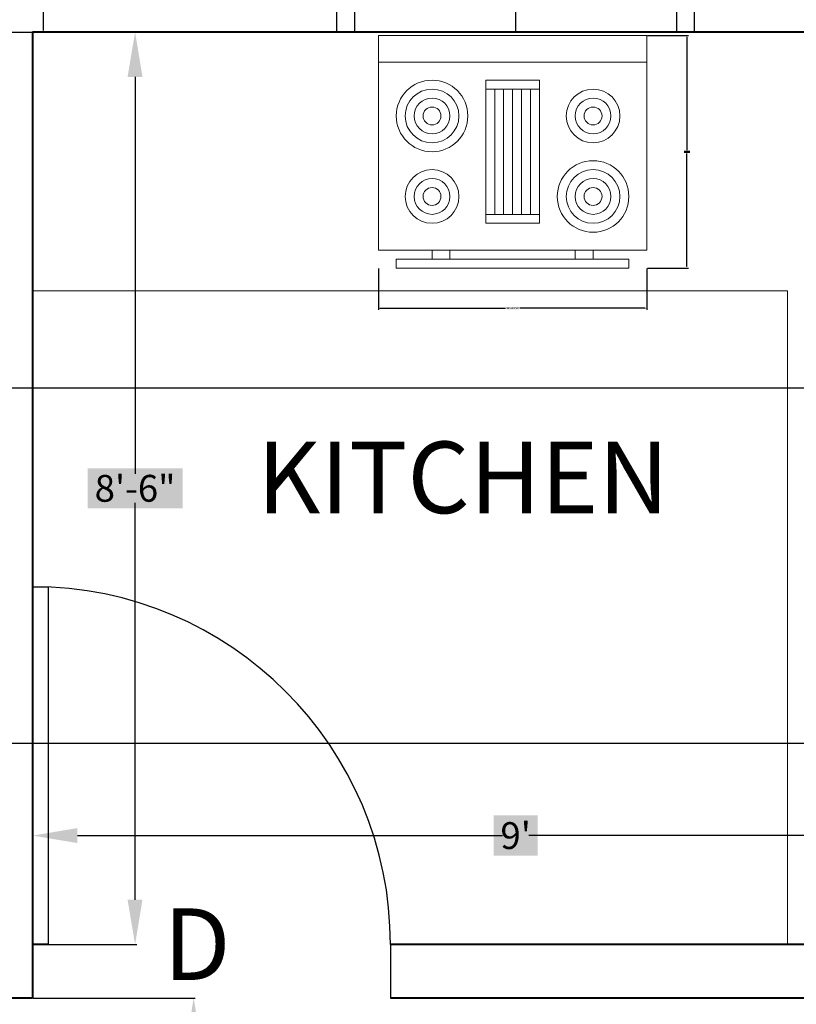
# Model space of a CAD drawing. Units: inches. Extents: x -301 to 715, y -607 to 364.
# Tile 118 of 141: x 14 to 101, y 192 to 303. Entities that reach past the tile are written whole.
import ezdxf

# ---------------------------------------------------------------- set-up
doc = ezdxf.new("R2010")
doc.units = ezdxf.units.IN
doc.header["$MEASUREMENT"] = 0
for name, color, linetype, lineweight in [('A-ANNO-DIMS', 2, 'Continuous', 18), ('A-ANNO-TEXT', 4, 'Continuous', 18), ('A-AREA-IDEN', 220, 'Continuous', 25), ('A-DOOR', 4, 'Continuous', 25), ('A-EQPM', 8, 'Continuous', 18), ('A-FLOR-CASE', 8, 'Continuous', 18), ('A-GLAZ', 2, 'Continuous', 25), ('A-WALL', 3, 'Continuous', 40)]:
    doc.layers.add(name, color=color, linetype=linetype, lineweight=lineweight)
doc.styles.get("Standard").update_dxf_attribs({"font": 'arial.ttf'})
doc.dimstyles.get("Standard").update_dxf_attribs({"dimtxt": 0.18, "dimasz": 0.18, "dimexe": 0.18, "dimexo": 0.0625, "dimgap": 0.09, "dimtad": 0, "dimtih": 1, "dimtoh": 1, "dimdec": 1, "dimzin": 0, "dimdsep": 46, "dimlunit": 4, "dimtxsty": 'Standard', "dimcen": 0.09, "dimclrd": 3, "dimclre": 4, "dimclrt": 6, "dimadec": 0, "dimazin": 0, "dimtfac": 1, "dimtdec": 1, "dimtofl": 0, "dimtmove": 0, "dimatfit": 3, "dimfxl": 1, "dimtfill": 2, "dimtfillclr": 51, "dimtolj": 1, "dimtzin": 0, "dimarcsym": 0})

# ---------------------------------------------------------------- blocks, each defined once
blk = doc.blocks.new('*U6')
for p, q in [((0, 0), (0, -6)), ((40, 0), (40, -6))]:
    blk.add_line(p, q)
blk.add_lwpolyline([(0, 0), (0, 40), (1.75, 40), (1.75, 0)], close=True)
blk.add_arc((0, 0), 40, 0, 90)
blk = doc.blocks.new('Range-Oven - 30 in top')
for p, q in [((0, -3), (30, -3)), ((12, -6), (18, -6)), ((13, -20), (13, -6)), ((14, -6), (14, -20)), ((15, -20), (15, -6)), ((16, -6), (16, -20)), ((17, -20), (17, -6)), ((18, -20), (12, -20)), ((6, -24), (6, -25)), ((8, -25), (8, -24)), ((22, -25), (22, -24)), ((24, -24), (24, -25))]:
    blk.add_line(p, q)
for points in [[(0, -24), (0, 0), (30, 0), (30, -24)], [(12, -21), (12, -5), (18, -5), (18, -21)], [(2, -26), (2, -25), (28, -25), (28, -26)]]:
    blk.add_lwpolyline(points, close=True)
for centre, radius in [((6, -9), 4), ((6, -9), 3), ((24, -9), 3), ((6, -9), 2), ((24, -9), 2), ((6, -9), 1), ((24, -9), 1), ((24, -18), 4), ((6, -18), 3), ((24, -18), 3), ((6, -18), 2), ((24, -18), 2), ((6, -18), 1), ((24, -18), 1)]:
    blk.add_circle(centre, radius)
blk = doc.blocks.new('*D49')
at = {"layer": 'A-ANNO-DIMS', "color": 0, "lineweight": -2, "transparency": 16777216}
for p, q in [((15.96, 193.18), (34.08, 193.18)), ((33.9, 188.18), (33.9, 93.3)), ((33.9, -4.82), (33.9, 90.06)), ((21.96, -9.82), (34.08, -9.82))]:
    blk.add_line(p, q, dxfattribs=at)
at = {"layer": 'A-ANNO-DIMS', "color": 0, "transparency": 16777216}
for points in [[(33.07, 188.18), (34.74, 188.18), (33.9, 193.18)], [(33.07, -4.82), (34.74, -4.82), (33.9, -9.82)]]:
    blk.add_solid(points, dxfattribs=at)
at = {"layer": 'Defpoints', "color": 0, "transparency": 16777216}
for p in [(15.9, 193.18), (33.9, 193.18), (21.9, -9.82)]:
    blk.add_point(p, dxfattribs=at)
at = {"layer": 'A-ANNO-DIMS', "color": 0, "transparency": 16777216, "insert": (33.9, 91.68), "char_height": 3, "attachment_point": 5, "bg_fill": 1, "box_fill_scale": 1.25, "bg_fill_color": 51, "bg_fill_transparency": 0}
blk.add_mtext('\\A1;16\'-11"', dxfattribs=at)
blk = doc.blocks.new('*D50')
at = {"layer": 'A-ANNO-DIMS', "color": 0, "lineweight": -2, "transparency": 16777216}
for p, q in [((15.9, 199.83), (15.9, 211.53)), ((123.9, 199.24), (123.9, 211.53)), ((20.9, 211.35), (68.43, 211.35)), ((118.9, 211.35), (71.37, 211.35))]:
    blk.add_line(p, q, dxfattribs=at)
at = {"layer": 'A-ANNO-DIMS', "color": 0, "transparency": 16777216}
for points in [[(20.9, 212.19), (20.9, 210.52), (15.9, 211.35)], [(118.9, 212.19), (118.9, 210.52), (123.9, 211.35)]]:
    blk.add_solid(points, dxfattribs=at)
at = {"layer": 'Defpoints', "color": 0, "transparency": 16777216}
for p in [(15.9, 211.35), (15.9, 199.77), (123.9, 199.18)]:
    blk.add_point(p, dxfattribs=at)
at = {"layer": 'A-ANNO-DIMS', "color": 0, "transparency": 16777216, "insert": (69.9, 211.35), "char_height": 3, "attachment_point": 5, "bg_fill": 1, "box_fill_scale": 1.25, "bg_fill_color": 51, "bg_fill_transparency": 0}
blk.add_mtext("\\A1;9'", dxfattribs=at)
blk = doc.blocks.new('*D51')
at = {"layer": 'A-ANNO-DIMS', "color": 0, "lineweight": -2, "transparency": 16777216}
for p, q in [((15.96, 301.18), (27.53, 301.18)), ((27.35, 296.18), (27.35, 251.8)), ((27.35, 204.18), (27.35, 248.56)), ((15.96, 199.18), (27.53, 199.18))]:
    blk.add_line(p, q, dxfattribs=at)
at = {"layer": 'A-ANNO-DIMS', "color": 0, "transparency": 16777216}
for points in [[(26.51, 296.18), (28.18, 296.18), (27.35, 301.18)], [(26.51, 204.18), (28.18, 204.18), (27.35, 199.18)]]:
    blk.add_solid(points, dxfattribs=at)
at = {"layer": 'Defpoints', "color": 0, "transparency": 16777216}
for p in [(15.9, 301.18), (15.9, 199.18), (27.35, 199.18)]:
    blk.add_point(p, dxfattribs=at)
at = {"layer": 'A-ANNO-DIMS', "color": 0, "transparency": 16777216, "insert": (27.35, 250.18), "char_height": 3, "attachment_point": 5, "bg_fill": 1, "box_fill_scale": 1.25, "bg_fill_color": 51, "bg_fill_transparency": 0}
blk.add_mtext('\\A1;8\'-6"', dxfattribs=at)
blk = doc.blocks.new('WIN-36-PLAN')
for p, q in [((0, 0), (0, 9)), ((2, 0), (2, 9)), ((20, 0), (20, 9)), ((38, 0), (38, 9)), ((40, 0), (40, 9)), ((2, 5.5), (38, 5.5)), ((2, 3.5), (38, 3.5))]:
    blk.add_line(p, q)
blk = doc.blocks.new('*D123')
at = {"layer": 'A-ANNO-DIMS', "color": 4, "lineweight": -2, "transparency": 16777216}
for p, q in [((9.96, 328.18), (17.28, 328.18)), ((9.96, 301.18), (17.28, 301.18))]:
    blk.add_line(p, q, dxfattribs=at)
at = {"layer": 'A-ANNO-DIMS', "color": 3, "lineweight": -2, "transparency": 16777216}
for p, q in [((17.1, 328), (17.1, 314.86)), ((17.1, 301.36), (17.1, 314.5))]:
    blk.add_line(p, q, dxfattribs=at)
at = {"layer": 'A-ANNO-DIMS', "color": 3, "transparency": 16777216}
for points in [[(17.07, 328), (17.13, 328), (17.1, 328.18)], [(17.07, 301.36), (17.13, 301.36), (17.1, 301.18)]]:
    blk.add_solid(points, dxfattribs=at)
at = {"layer": 'Defpoints', "color": 0, "transparency": 16777216}
for p in [(9.9, 328.18), (9.9, 301.18), (17.1, 301.18)]:
    blk.add_point(p, dxfattribs=at)
at = {"layer": 'A-ANNO-DIMS', "color": 6, "transparency": 16777216, "insert": (17.1, 314.68), "char_height": 0.18, "attachment_point": 5, "bg_fill": 1, "box_fill_scale": 1.25, "bg_fill_color": 51, "bg_fill_transparency": 0}
blk.add_mtext('\\A1;2\'-3" TYP.', dxfattribs=at)
blk = doc.blocks.new('*D140')
at = {"layer": 'A-ANNO-DIMS', "color": 4, "lineweight": -2, "transparency": 16777216}
for p, q in [((54.55, 274.74), (54.55, 270.13)), ((84.55, 274.74), (84.55, 270.13))]:
    blk.add_line(p, q, dxfattribs=at)
at = {"layer": 'A-ANNO-DIMS', "color": 3, "lineweight": -2, "transparency": 16777216}
for p, q in [((54.73, 270.31), (68.75, 270.31)), ((84.37, 270.31), (70.36, 270.31))]:
    blk.add_line(p, q, dxfattribs=at)
at = {"layer": 'A-ANNO-DIMS', "color": 3, "transparency": 16777216}
for points in [[(54.73, 270.34), (54.73, 270.28), (54.55, 270.31)], [(84.37, 270.34), (84.37, 270.28), (84.55, 270.31)]]:
    blk.add_solid(points, dxfattribs=at)
at = {"layer": 'Defpoints', "color": 0, "transparency": 16777216}
for p in [(54.55, 274.81), (84.55, 274.81), (84.55, 270.31)]:
    blk.add_point(p, dxfattribs=at)
at = {"layer": 'A-ANNO-DIMS', "color": 6, "transparency": 16777216, "insert": (69.55, 270.31), "char_height": 0.18, "attachment_point": 5, "bg_fill": 1, "box_fill_scale": 1.25, "bg_fill_color": 51, "bg_fill_transparency": 0}
blk.add_mtext('\\A1;RANGE 2\'-6"', dxfattribs=at)
blk = doc.blocks.new('*D141')
at = {"layer": 'A-ANNO-DIMS', "color": 4, "lineweight": -2, "transparency": 16777216}
for p, q in [((84.62, 300.81), (89.23, 300.81)), ((84.62, 274.81), (89.23, 274.81))]:
    blk.add_line(p, q, dxfattribs=at)
at = {"layer": 'A-ANNO-DIMS', "color": 3, "lineweight": -2, "transparency": 16777216}
for p, q in [((89.05, 300.63), (89.05, 287.99)), ((89.05, 274.99), (89.05, 287.63))]:
    blk.add_line(p, q, dxfattribs=at)
at = {"layer": 'A-ANNO-DIMS', "color": 3, "transparency": 16777216}
for points in [[(89.02, 300.63), (89.08, 300.63), (89.05, 300.81)], [(89.02, 274.99), (89.08, 274.99), (89.05, 274.81)]]:
    blk.add_solid(points, dxfattribs=at)
at = {"layer": 'Defpoints', "color": 0, "transparency": 16777216}
for p in [(84.55, 300.81), (89.05, 300.81), (84.55, 274.81)]:
    blk.add_point(p, dxfattribs=at)
at = {"layer": 'A-ANNO-DIMS', "color": 6, "transparency": 16777216, "insert": (89.05, 287.81), "char_height": 0.18, "attachment_point": 5, "bg_fill": 1, "box_fill_scale": 1.25, "bg_fill_color": 51, "bg_fill_transparency": 0}
blk.add_mtext('\\A1;2\'-2"', dxfattribs=at)
blk = doc.blocks.new('*D157')
at = {"layer": 'A-ANNO-DIMS', "color": 4, "lineweight": -2, "transparency": 16777216}
for p, q in [((-50.54, 261.43), (233.66, 261.43)), ((-50.54, 221.68), (233.66, 221.68))]:
    blk.add_line(p, q, dxfattribs=at)
at = {"layer": 'A-ANNO-DIMS', "color": 3, "lineweight": -2, "transparency": 16777216}
for p, q in [((233.48, 261.25), (233.48, 241.74)), ((233.48, 221.86), (233.48, 241.38))]:
    blk.add_line(p, q, dxfattribs=at)
at = {"layer": 'A-ANNO-DIMS', "color": 3, "transparency": 16777216}
for points in [[(233.45, 261.25), (233.51, 261.25), (233.48, 261.43)], [(233.45, 221.86), (233.51, 221.86), (233.48, 221.68)]]:
    blk.add_solid(points, dxfattribs=at)
at = {"layer": 'Defpoints', "color": 0, "transparency": 16777216}
for p in [(-50.6, 261.43), (233.48, 261.43), (-50.6, 221.68)]:
    blk.add_point(p, dxfattribs=at)
at = {"layer": 'A-ANNO-DIMS', "color": 6, "transparency": 16777216, "insert": (233.48, 241.56), "char_height": 0.18, "attachment_point": 5, "bg_fill": 1, "box_fill_scale": 1.25, "bg_fill_color": 51, "bg_fill_transparency": 0}
blk.add_mtext('\\A1;3\'-4"', dxfattribs=at)

msp = doc.modelspace()

# ---------------------------------------------------------------- linework, layer by layer
at = {"layer": 'A-FLOR-CASE'}
for p, q in [((15.9, 272.26), (100.3, 272.26)), ((100.3, 272.26), (100.3, 199.18))]:
    msp.add_line(p, q, dxfattribs=at)
at = {"layer": 'A-WALL'}
for p, q in [((123.9, 301.18), (15.9, 301.18)), ((15.9, 301.18), (15.9, 193.18)), ((17.65, 199.18), (15.9, 199.18)), ((123.9, 199.18), (55.9, 199.18)), ((15.9, 193.18), (9.9, 193.18)), ((123.9, 193.18), (55.9, 193.18))]:
    msp.add_line(p, q, dxfattribs=at)

# ---------------------------------------------------------------- block references
at = {"layer": 'A-DOOR'}
msp.add_blockref('*U6', (15.9, 199.18), dxfattribs=at)
at = {"layer": 'A-EQPM'}
msp.add_blockref('Range-Oven - 30 in top', (54.55, 300.81), dxfattribs=at)
at = {"layer": 'A-GLAZ'}
msp.add_blockref('WIN-36-PLAN', (49.9, 301.18), dxfattribs=at)

# ---------------------------------------------------------------- texts
at = {"layer": 'A-ANNO-TEXT'}
msp.add_text('D', height=8, dxfattribs=at).set_placement((30.52, 195.21))
at = {"layer": 'A-AREA-IDEN', "insert": (41.01, 255.4), "char_height": 8, "attachment_point": 1}
msp.add_mtext_dynamic_manual_height_columns('KITCHEN', width=73.06, gutter_width=1, heights=[0], dxfattribs=at)

# ---------------------------------------------------------------- dimensions: what is measured, and where the dimension line sits
at = {"layer": 'A-ANNO-DIMS'}
dim = msp.add_linear_dim(base=(17.1, 301.18), p1=(9.9, 328.18), p2=(9.9, 301.18), angle=270, text='<> TYP.', dimstyle='Standard', override={"dimdec": 1, "dimlfac": 1, "dimrnd": 0, "dimzin": 1, "dimdsep": 46, "dimlunit": 4, "dimfrac": 2}, dxfattribs=at)
dim.commit()
dim.dimension.update_dxf_attribs({"geometry": '*D123', "text_midpoint": (17.1, 314.68)})
for base, p1, p2, override, picture, middle in [((27.35, 199.18), (15.9, 301.18), (15.9, 199.18), {"dimtxt": 3, "dimasz": 5, "dimclrd": 0, "dimclre": 0, "dimclrt": 0}, '*D51', (27.35, 250.18)), ((89.05, 300.81), (84.55, 274.81), (84.55, 300.81), {"dimdec": 1, "dimlfac": 1, "dimrnd": 0, "dimzin": 1, "dimdsep": 46, "dimlunit": 4, "dimfrac": 2}, '*D141', (89.05, 287.81)), ((233.479242, 261.43233), (-50.603288, 221.68233), (-50.603288, 261.43233), {"dimdec": 1, "dimlfac": 1, "dimrnd": 0, "dimzin": 1, "dimdsep": 46, "dimlunit": 4, "dimfrac": 2}, '*D157', (233.479242, 241.55733)), ((33.9, 193.18), (21.9, -9.82), (15.9, 193.18), {"dimtxt": 3, "dimasz": 5, "dimclrd": 0, "dimclre": 0, "dimclrt": 0}, '*D49', (33.9, 91.68))]:
    dim = msp.add_linear_dim(base=base, p1=p1, p2=p2, angle=90, dimstyle='Standard', override=override, dxfattribs=at)
    dim.commit()
    dim.dimension.update_dxf_attribs({"geometry": picture, "text_midpoint": middle})
dim = msp.add_linear_dim(base=(84.55, 270.31), p1=(54.55, 274.81), p2=(84.55, 274.81), text='RANGE <>', dimstyle='Standard', override={"dimdec": 1, "dimlfac": 1, "dimrnd": 0, "dimzin": 1, "dimdsep": 46, "dimlunit": 4, "dimfrac": 2}, dxfattribs=at)
dim.commit()
dim.dimension.update_dxf_attribs({"geometry": '*D140', "text_midpoint": (69.55, 270.31)})
dim = msp.add_linear_dim(base=(15.9, 211.35), p1=(123.9, 199.18), p2=(15.9, 199.77), dimstyle='Standard', override={"dimtxt": 3, "dimasz": 5, "dimclrd": 0, "dimclre": 0, "dimclrt": 0}, dxfattribs=at)
dim.commit()
dim.dimension.update_dxf_attribs({"geometry": '*D50', "text_midpoint": (69.9, 211.35)})

doc.saveas('drawing.dxf')
